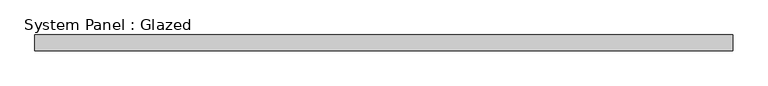
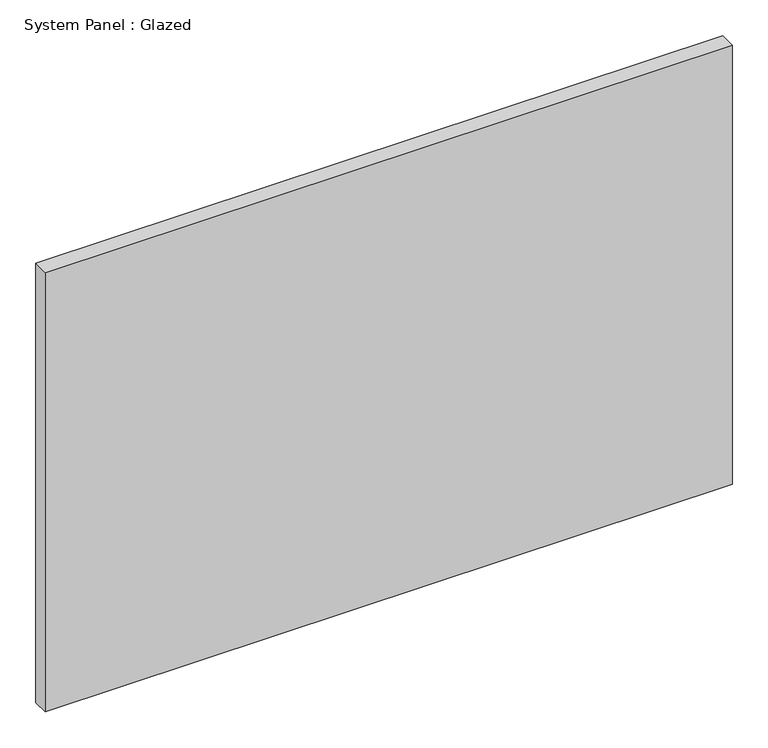
"""IFC4 building model written with IfcOpenShell, lengths in millimetres: plate geometry, System Panel : Glazed."""

from ifc_helpers import new_model, si_unit, origin, origin_with_axes, place, context, project, spatial, polyline, outline, extrude, source, transform, mapped, element, save


def system_panel_glazed_b873dfd1(model_context):
    return source(origin(), model_context, "Body", "SweptSolid", [
        extrude(outline(polyline([(551.392122, 19.05), (-551.392122, 19.05), (-551.392122, 44.45), (551.392122, 44.45), (551.392122, 19.05)])), origin_with_axes(), (0.0, 0.0, 1.0), 745.7790241),
    ])


if __name__ == "__main__":
    model = new_model("IFC4")
    model_context = context("Model", 3, world=origin())
    ifc_project = project(units=[si_unit("LENGTHUNIT", "METRE", prefix="MILLI")], contexts=[model_context])
    site = spatial("IfcSite", under=ifc_project)
    building = spatial("IfcBuilding", under=site)
    placement = place(None, origin())
    system_panel_glazed_shape = system_panel_glazed_b873dfd1(model_context)
    element("IfcPlate", 1, ObjectType="System Panel : Glazed", at=placement, inside=building, context=model_context, shape_type="MappedRepresentation", body=[
        mapped(system_panel_glazed_shape, transform((0.0, 0.0, 0.0), x_axis=(1.0, 0.0, 0.0), y_axis=(0.0, 1.0, 0.0), z_axis=(0.0, 0.0, 1.0))),
    ])
    save(model, "model.ifc")

# Revit data of these elements
# Type "System Panel : Glazed"
#   Construction Type Id = "GSP4R"
#   Analytic Construction = "1/8 in Pilkington single glazing"
#   Visual Light Transmittance = 0.9
#   Solar Heat Gain Coefficient = 0.86
#   Heat Transfer Coefficient (U) = 1.18115 BTU/(h·ft²·°F)
# Element 1 (IfcPlate, "System Panel : Glazed")
#   Materials on its faces: "Glass"
# Materials
#   "Glass": class "Glass", colour RGB 0 128 192, transparency 0.75, Description = "Soda Lime Glass", Cost = 0
